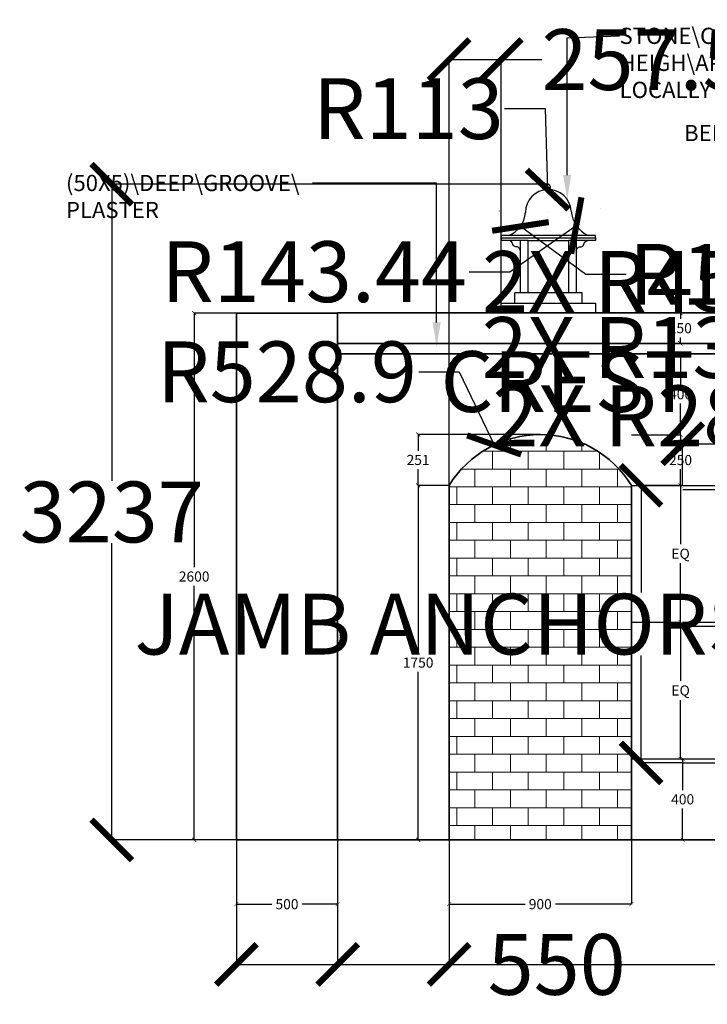
# Model space of a CAD drawing. Units: millimetres. Extents: x 16635 to 28332, y 17519 to 22633.
# Tile 1 of 4: x 16635 to 20029, y 17772 to 22633. Entities that reach past the tile are written whole.
import ezdxf
from ezdxf import colors
from ezdxf.entities.mleader import LeaderData, LeaderLine
from ezdxf.math import Vec2, Vec3

# ---------------------------------------------------------------- set-up
doc = ezdxf.new("R2010")
doc.units = ezdxf.units.MM
doc.header["$MEASUREMENT"] = 0
for name, color, linetype, lineweight in [('A-ANNO-DIMS', 2, 'Continuous', 18), ('A-ANNO-TEXT', 7, 'Continuous', 18), ('A-GATE-HRDW', 3, 'Continuous', 25), ('A-WALL', 7, 'Continuous', 35), ('A-WALL-CHTR', 32, 'Continuous', 25), ('A-WALL-PATT', 8, 'Continuous', 13)]:
    doc.layers.add(name, color=color, linetype=linetype, lineweight=lineweight)
doc.styles.get("Standard").update_dxf_attribs({"font": 'arial.ttf'})
doc.dimstyles.get("Standard").update_dxf_attribs({"dimtxt": 300, "dimasz": 200, "dimexe": 0.18, "dimexo": 0.0625, "dimgap": 0.09, "dimtad": 0, "dimtih": 1, "dimtoh": 1, "dimdec": 0, "dimzin": 0, "dimdsep": 46, "dimtxsty": 'Standard', "dimblk": 'ARCHTICK', "dimcen": 0.09, "dimadec": 0, "dimazin": 0, "dimtfac": 1, "dimtdec": 0, "dimtofl": 0, "dimtmove": 0, "dimatfit": 3, "dimfxl": 1, "dimtolj": 1, "dimtzin": 0, "dimarcsym": 0})

# ---------------------------------------------------------------- blocks, each defined once
blk = doc.blocks.new('_ArchTick')
at = {"color": 0, "linetype": 'ByBlock', "const_width": 0.15}
blk.add_lwpolyline([(-0.5, -0.5), (0.5, 0.5)], dxfattribs=at)
blk = doc.blocks.new('*D9')
at = {"layer": 'A-ANNO-DIMS', "color": 0, "lineweight": -2, "transparency": 16777216}
for p, q in [((18754.7, 20334.3), (18601.7, 20334.3)), ((18601.9, 20334.3), (18601.9, 19504.9)), ((18601.9, 18584.3), (18601.9, 19413.8)), ((18754.7, 18584.3), (18601.7, 18584.3))]:
    blk.add_line(p, q, dxfattribs=at)
at = {"layer": 'Defpoints', "color": 0, "transparency": 16777216}
for p in [(18754.8, 20334.3), (18601.9, 18584.3), (18754.8, 18584.3)]:
    blk.add_point(p, dxfattribs=at)
at = {"layer": 'A-ANNO-DIMS', "color": 0, "lineweight": -2, "transparency": 16777216, "xscale": 20, "yscale": 20, "zscale": 20}
for p, rotation in [((18601.9, 20334.3), 90), ((18601.9, 18584.3), 270)]:
    blk.add_blockref('_ArchTick', p, dxfattribs=dict(at, rotation=rotation))
at = {"layer": 'A-ANNO-DIMS', "color": 0, "transparency": 16777216, "insert": (18601.9, 19459.3), "char_height": 50, "attachment_point": 5}
blk.add_mtext('\\A1;1750', dxfattribs=at)
blk = doc.blocks.new('*D10')
at = {"layer": 'A-ANNO-DIMS', "color": 0, "lineweight": -2, "transparency": 16777216}
for p, q in [((19204.7, 20585.3), (18601.7, 20585.3)), ((18601.9, 20585.3), (18601.9, 20505.4)), ((18601.9, 20334.3), (18601.9, 20414.3)), ((18754.7, 20334.3), (18601.7, 20334.3))]:
    blk.add_line(p, q, dxfattribs=at)
at = {"layer": 'Defpoints', "color": 0, "transparency": 16777216}
for p in [(18601.9, 20585.3), (19204.8, 20585.3), (18754.8, 20334.3)]:
    blk.add_point(p, dxfattribs=at)
at = {"layer": 'A-ANNO-DIMS', "color": 0, "lineweight": -2, "transparency": 16777216, "xscale": 20, "yscale": 20, "zscale": 20}
for p, rotation in [((18601.9, 20585.3), 90), ((18601.9, 20334.3), 270)]:
    blk.add_blockref('_ArchTick', p, dxfattribs=dict(at, rotation=rotation))
at = {"layer": 'A-ANNO-DIMS', "color": 0, "transparency": 16777216, "insert": (18601.9, 20459.8), "char_height": 50, "attachment_point": 5}
blk.add_mtext('\\A1;251', dxfattribs=at)
blk = doc.blocks.new('*D11')
at = {"layer": 'A-ANNO-DIMS', "color": 0, "lineweight": -2, "transparency": 16777216}
for p, q in [((19654.8, 20584.3), (19897.4, 20584.3)), ((19897.2, 20584.3), (19897.2, 20504.9)), ((19897.2, 20334.3), (19897.2, 20413.8)), ((19654.8, 20334.3), (19897.4, 20334.3))]:
    blk.add_line(p, q, dxfattribs=at)
at = {"layer": 'Defpoints', "color": 0, "transparency": 16777216}
for p in [(19654.8, 20584.3), (19897.2, 20584.3), (19654.8, 20334.3)]:
    blk.add_point(p, dxfattribs=at)
at = {"layer": 'A-ANNO-DIMS', "color": 0, "lineweight": -2, "transparency": 16777216, "xscale": 20, "yscale": 20, "zscale": 20}
for p, rotation in [((19897.2, 20584.3), 90), ((19897.2, 20334.3), 270)]:
    blk.add_blockref('_ArchTick', p, dxfattribs=dict(at, rotation=rotation))
at = {"layer": 'A-ANNO-DIMS', "color": 0, "transparency": 16777216, "insert": (19897.2, 20459.3), "char_height": 50, "attachment_point": 5}
blk.add_mtext('\\A1;250', dxfattribs=at)
blk = doc.blocks.new('*D12')
at = {"layer": 'A-ANNO-DIMS', "color": 0, "lineweight": -2, "transparency": 16777216}
for p, q in [((19654.8, 20984.3), (19897.6, 20984.3)), ((19897.4, 20984.3), (19897.4, 20829.9)), ((19897.4, 20584.3), (19897.4, 20738.8)), ((19654.8, 20584.3), (19897.6, 20584.3))]:
    blk.add_line(p, q, dxfattribs=at)
at = {"layer": 'Defpoints', "color": 0, "transparency": 16777216}
for p in [(19654.8, 20984.3), (19897.4, 20984.3), (19654.8, 20584.3)]:
    blk.add_point(p, dxfattribs=at)
at = {"layer": 'A-ANNO-DIMS', "color": 0, "lineweight": -2, "transparency": 16777216, "xscale": 20, "yscale": 20, "zscale": 20}
for p, rotation in [((19897.4, 20984.3), 90), ((19897.4, 20584.3), 270)]:
    blk.add_blockref('_ArchTick', p, dxfattribs=dict(at, rotation=rotation))
at = {"layer": 'A-ANNO-DIMS', "color": 0, "transparency": 16777216, "insert": (19897.4, 20784.3), "char_height": 50, "attachment_point": 5}
blk.add_mtext('\\A1;400', dxfattribs=at)
blk = doc.blocks.new('*D18')
at = {"layer": 'A-ANNO-DIMS', "color": 0, "lineweight": -2, "transparency": 16777216}
for p, q in [((17704.7, 21184.3), (17496.3, 21184.3)), ((17496.5, 21184.3), (17496.5, 19929.9)), ((17496.5, 18584.3), (17496.5, 19838.8)), ((17704.7, 18584.3), (17496.3, 18584.3))]:
    blk.add_line(p, q, dxfattribs=at)
at = {"layer": 'Defpoints', "color": 0, "transparency": 16777216}
for p in [(17704.8, 21184.3), (17496.5, 18584.3), (17704.8, 18584.3)]:
    blk.add_point(p, dxfattribs=at)
at = {"layer": 'A-ANNO-DIMS', "color": 0, "lineweight": -2, "transparency": 16777216, "xscale": 20, "yscale": 20, "zscale": 20}
for p, rotation in [((17496.5, 21184.3), 90), ((17496.5, 18584.3), 270)]:
    blk.add_blockref('_ArchTick', p, dxfattribs=dict(at, rotation=rotation))
at = {"layer": 'A-ANNO-DIMS', "color": 0, "transparency": 16777216, "insert": (17496.5, 19884.3), "char_height": 50, "attachment_point": 5}
blk.add_mtext('\\A1;2600', dxfattribs=at)
blk = doc.blocks.new('*D23')
at = {"layer": 'A-ANNO-DIMS', "color": 0, "lineweight": -2, "transparency": 16777216}
for p, q in [((18754.8, 18584.3), (18754.8, 18266.8)), ((19654.8, 18584.3), (19654.8, 18266.8)), ((18754.8, 18267), (19129.6, 18267)), ((19654.8, 18267), (19279.9, 18267))]:
    blk.add_line(p, q, dxfattribs=at)
at = {"layer": 'Defpoints', "color": 0, "transparency": 16777216}
for p in [(18754.8, 18584.3), (19654.8, 18584.3), (19654.8, 18267)]:
    blk.add_point(p, dxfattribs=at)
at = {"layer": 'A-ANNO-DIMS', "color": 0, "lineweight": -2, "transparency": 16777216, "xscale": 20, "yscale": 20, "zscale": 20, "rotation": 180}
blk.add_blockref('_ArchTick', (18754.8, 18267), dxfattribs=at)
at = {"layer": 'A-ANNO-DIMS', "color": 0, "lineweight": -2, "transparency": 16777216, "xscale": 20, "yscale": 20, "zscale": 20}
blk.add_blockref('_ArchTick', (19654.8, 18267), dxfattribs=at)
at = {"layer": 'A-ANNO-DIMS', "color": 0, "transparency": 16777216, "insert": (19204.8, 18267), "char_height": 50, "attachment_point": 5}
blk.add_mtext('\\A1;900', dxfattribs=at)
blk = doc.blocks.new('*D24')
at = {"layer": 'A-ANNO-DIMS', "color": 0, "lineweight": -2, "transparency": 16777216}
for p, q in [((17704.8, 18584.3), (17704.8, 18266.6)), ((18204.8, 18584.3), (18204.8, 18266.6)), ((17704.8, 18266.8), (17879.6, 18266.8)), ((18204.8, 18266.8), (18029.9, 18266.8))]:
    blk.add_line(p, q, dxfattribs=at)
at = {"layer": 'Defpoints', "color": 0, "transparency": 16777216}
for p in [(17704.8, 18584.3), (18204.8, 18584.3), (18204.8, 18266.8)]:
    blk.add_point(p, dxfattribs=at)
at = {"layer": 'A-ANNO-DIMS', "color": 0, "lineweight": -2, "transparency": 16777216, "xscale": 20, "yscale": 20, "zscale": 20, "rotation": 180}
blk.add_blockref('_ArchTick', (17704.8, 18266.8), dxfattribs=at)
at = {"layer": 'A-ANNO-DIMS', "color": 0, "lineweight": -2, "transparency": 16777216, "xscale": 20, "yscale": 20, "zscale": 20}
blk.add_blockref('_ArchTick', (18204.8, 18266.8), dxfattribs=at)
at = {"layer": 'A-ANNO-DIMS', "color": 0, "transparency": 16777216, "insert": (17954.8, 18266.8), "char_height": 50, "attachment_point": 5}
blk.add_mtext('\\A1;500', dxfattribs=at)
blk = doc.blocks.new('*D31')
at = {"layer": 'A-ANNO-DIMS', "color": 0, "lineweight": -2, "transparency": 16777216}
for p, q in [((19654.8, 18984.3), (19907.7, 18984.3)), ((19907.6, 18984.3), (19907.6, 18829.9)), ((19907.6, 18584.3), (19907.6, 18738.8)), ((19654.8, 18584.3), (19907.7, 18584.3))]:
    blk.add_line(p, q, dxfattribs=at)
at = {"layer": 'Defpoints', "color": 0, "transparency": 16777216}
for p in [(19654.8, 18984.3), (19907.6, 18984.3), (19654.8, 18584.3)]:
    blk.add_point(p, dxfattribs=at)
at = {"layer": 'A-ANNO-DIMS', "color": 0, "lineweight": -2, "transparency": 16777216, "xscale": 20, "yscale": 20, "zscale": 20}
for p, rotation in [((19907.6, 18984.3), 90), ((19907.6, 18584.3), 270)]:
    blk.add_blockref('_ArchTick', p, dxfattribs=dict(at, rotation=rotation))
at = {"layer": 'A-ANNO-DIMS', "color": 0, "transparency": 16777216, "insert": (19907.6, 18784.3), "char_height": 50, "attachment_point": 5}
blk.add_mtext('\\A1;400', dxfattribs=at)
blk = doc.blocks.new('*D35')
at = {"layer": 'A-ANNO-DIMS', "color": 0, "lineweight": -2, "transparency": 16777216}
for p, q in [((19654.8, 20334.3), (19897.6, 20334.3)), ((19897.4, 20334.3), (19897.4, 20044.2)), ((19897.4, 19659.3), (19897.4, 19949.5)), ((19654.8, 19659.3), (19897.6, 19659.3))]:
    blk.add_line(p, q, dxfattribs=at)
at = {"layer": 'Defpoints', "color": 0, "transparency": 16777216}
for p in [(19654.8, 20334.3), (19654.8, 19659.3), (19897.4, 19659.3)]:
    blk.add_point(p, dxfattribs=at)
at = {"layer": 'A-ANNO-DIMS', "color": 0, "lineweight": -2, "transparency": 16777216, "xscale": 20, "yscale": 20, "zscale": 20}
for p, rotation in [((19897.4, 20334.3), 90), ((19897.4, 19659.3), 270)]:
    blk.add_blockref('_ArchTick', p, dxfattribs=dict(at, rotation=rotation))
at = {"layer": 'A-ANNO-DIMS', "color": 0, "transparency": 16777216, "insert": (19897.4, 19996.8), "char_height": 50, "attachment_point": 5}
blk.add_mtext('\\A1;EQ', dxfattribs=at)
blk = doc.blocks.new('*D36')
at = {"layer": 'A-ANNO-DIMS', "color": 0, "lineweight": -2, "transparency": 16777216}
for p, q in [((19654.8, 19659.3), (19897.7, 19659.3)), ((19897.6, 19659.3), (19897.6, 19369.2)), ((19897.6, 18984.3), (19897.6, 19274.5)), ((19654.8, 18984.3), (19897.7, 18984.3))]:
    blk.add_line(p, q, dxfattribs=at)
at = {"layer": 'Defpoints', "color": 0, "transparency": 16777216}
for p in [(19654.8, 19659.3), (19654.8, 18984.3), (19897.6, 18984.3)]:
    blk.add_point(p, dxfattribs=at)
at = {"layer": 'A-ANNO-DIMS', "color": 0, "lineweight": -2, "transparency": 16777216, "xscale": 20, "yscale": 20, "zscale": 20}
for p, rotation in [((19897.6, 19659.3), 90), ((19897.6, 18984.3), 270)]:
    blk.add_blockref('_ArchTick', p, dxfattribs=dict(at, rotation=rotation))
at = {"layer": 'A-ANNO-DIMS', "color": 0, "transparency": 16777216, "insert": (19897.6, 19321.8), "char_height": 50, "attachment_point": 5}
blk.add_mtext('\\A1;EQ', dxfattribs=at)
blk = doc.blocks.new('*D37')
at = {"layer": 'A-ANNO-DIMS', "color": 0, "lineweight": -2, "transparency": 16777216}
for p, q in [((19896.2, 21185.3), (19896.2, 21155.9)), ((19896.3, 21185.3), (19896.4, 21185.3)), ((19896.2, 21035.3), (19896.2, 21064.8)), ((19896.3, 21035.3), (19896.4, 21035.3))]:
    blk.add_line(p, q, dxfattribs=at)
at = {"layer": 'Defpoints', "color": 0, "transparency": 16777216}
for p in [(19896.2, 21185.3), (19896.2, 21185.3), (19896.2, 21035.3)]:
    blk.add_point(p, dxfattribs=at)
at = {"layer": 'A-ANNO-DIMS', "color": 0, "lineweight": -2, "transparency": 16777216, "xscale": 20, "yscale": 20, "zscale": 20}
for p, rotation in [((19896.2, 21185.3), 90), ((19896.2, 21035.3), 270)]:
    blk.add_blockref('_ArchTick', p, dxfattribs=dict(at, rotation=rotation))
at = {"layer": 'A-ANNO-DIMS', "color": 0, "transparency": 16777216, "insert": (19896.2, 21110.3), "char_height": 50, "attachment_point": 5}
blk.add_mtext('\\A1;150', dxfattribs=at)
blk = doc.blocks.new('STONE-CHHATRI-ELEV')
for p, q in [((465, 384), (0, 384)), ((0, 384), (0, 359)), ((0, 371.5), (465, 371.5)), ((132.5, 359), (0, 359)), ((94.5, 100), (94.5, 359)), ((132.5, 100), (132.5, 359)), ((132.5, 359), (332.5, 359)), ((332.5, 359), (332.5, 100)), ((465, 359), (332.5, 359)), ((370.5, 359), (370.5, 100)), ((465, 371.5), (465, 384)), ((465, 371.5), (465, 359)), ((398.8, 100), (66.3, 100)), ((66.3, 50), (66.3, 100)), ((398.8, 50), (398.8, 100)), ((0, 0), (0, 50)), ((0, 50), (465, 50)), ((465, 50), (465, 0))]:
    blk.add_line(p, q)
for points in [[(223.5, 618.7, -0.258687), (233, 636.9, -0.244698), (241.5, 619.3, -0.244698)], [(94.5, 307.9, 0.449164), (70.8, 327.5, -0.238561), (57.7, 338.5, 0.309009), (37.1, 359, -1.219644)], [(370.5, 307.9, -0.449164), (394.2, 327.5, 0.238561), (407.3, 338.5, -0.309009), (427.9, 359, 1.219644)]]:
    blk.add_lwpolyline(points, format="xyb")
for centre, radius, start, end in [((232.5, 497), 113, 3.6245, 179.9064), ((232.5, 619), 9.02, 180.1799, 1.9928), ((-8.8, 504.3), 128.5, 290.6287, 356.8247), ((488.3, 514.4), 143.4, 184.0947, 245.367)]:
    blk.add_arc(centre, radius, start, end)
blk = doc.blocks.new('GATE-JAMB-ANCHOR-SET')
for p, q in [((0.2, 1370), (297.2, 1370)), ((317.2, 1350), (317.2, 1370)), ((317.2, 1370), (351.9, 1370)), ((0.2, 1350), (297.2, 1350)), ((297.2, 1350), (317.2, 1350)), ((0, 694.8), (297, 694.8)), ((317, 674.8), (317, 694.8)), ((317, 694.8), (365.3, 694.8)), ((0, 674.8), (297, 674.8)), ((297, 674.8), (317, 674.8)), ((0.2, 20), (297.2, 20)), ((317.2, 0), (317.2, 20)), ((317.2, 20), (360.9, 20)), ((0.2, 0), (297.2, 0)), ((297.2, 0), (317.2, 0))]:
    blk.add_line(p, q)
blk = doc.blocks.new('*D47')
at = {"layer": 'A-ANNO-DIMS', "color": 0, "lineweight": -2, "transparency": 16777216}
for p, q in [((21092.8, 21187.8), (20990.3, 21187.8)), ((20990.5, 21187.8), (20990.5, 21001.9)), ((20990.5, 20505.3), (20990.5, 20691.3)), ((21092.8, 20505.3), (20990.3, 20505.3))]:
    blk.add_line(p, q, dxfattribs=at)
at = {"layer": 'Defpoints', "color": 0, "transparency": 16777216}
for p in [(20990.5, 21187.8), (21092.8, 21187.8), (21092.8, 20505.3)]:
    blk.add_point(p, dxfattribs=at)
at = {"layer": 'A-ANNO-DIMS', "color": 0, "lineweight": -2, "transparency": 16777216, "xscale": 200, "yscale": 200, "zscale": 200}
for p, rotation in [((20990.5, 21187.8), 90), ((20990.5, 20505.3), 270)]:
    blk.add_blockref('_ArchTick', p, dxfattribs=dict(at, rotation=rotation))
at = {"layer": 'A-ANNO-DIMS', "color": 0, "transparency": 16777216, "insert": (20990.5, 20846.6), "char_height": 300, "attachment_point": 5}
blk.add_mtext('\\A1;CREST SCROLL 682 TYP.', dxfattribs=at)
blk = doc.blocks.new('*D49')
at = {"layer": 'A-ANNO-DIMS', "color": 0, "lineweight": -2, "transparency": 16777216}
for p, q in [((19907.5, 20334.3), (19701.9, 20334.3)), ((19702.1, 20334.3), (19702.1, 19804.8)), ((19702.1, 18964.3), (19702.1, 19493.9)), ((19907.5, 18964.3), (19701.9, 18964.3))]:
    blk.add_line(p, q, dxfattribs=at)
at = {"layer": 'Defpoints', "color": 0, "transparency": 16777216}
for p in [(19702.1, 20334.3), (19907.6, 20334.3), (19907.6, 18964.3)]:
    blk.add_point(p, dxfattribs=at)
at = {"layer": 'A-ANNO-DIMS', "color": 0, "lineweight": -2, "transparency": 16777216, "xscale": 200, "yscale": 200, "zscale": 200}
for p, rotation in [((19702.1, 20334.3), 90), ((19702.1, 18964.3), 270)]:
    blk.add_blockref('_ArchTick', p, dxfattribs=dict(at, rotation=rotation))
at = {"layer": 'A-ANNO-DIMS', "color": 0, "transparency": 16777216, "insert": (19702.1, 19649.3), "char_height": 300, "attachment_point": 5}
blk.add_mtext('\\A1;JAMB ANCHORS 1370 TYP.', dxfattribs=at)
blk = doc.blocks.new('*D50')
at = {"layer": 'A-ANNO-DIMS', "color": 0, "lineweight": -2, "transparency": 16777216}
for p, q in [((19907.6, 20334.4), (19907.6, 20540)), ((19907.6, 20539.8), (20272.8, 20539.8)), ((20272.8, 20334.4), (20272.8, 20540)), ((20272.8, 20539.8), (20472.8, 20539.8))]:
    blk.add_line(p, q, dxfattribs=at)
at = {"layer": 'Defpoints', "color": 0, "transparency": 16777216}
for p in [(20272.8, 20539.8), (19907.6, 20334.3), (20272.8, 20334.3)]:
    blk.add_point(p, dxfattribs=at)
at = {"layer": 'A-ANNO-DIMS', "color": 0, "lineweight": -2, "transparency": 16777216, "xscale": 200, "yscale": 200, "zscale": 200, "rotation": 180}
blk.add_blockref('_ArchTick', (19907.6, 20539.8), dxfattribs=at)
at = {"layer": 'A-ANNO-DIMS', "color": 0, "lineweight": -2, "transparency": 16777216, "xscale": 200, "yscale": 200, "zscale": 200}
blk.add_blockref('_ArchTick', (20272.8, 20539.8), dxfattribs=at)
at = {"layer": 'A-ANNO-DIMS', "color": 0, "transparency": 16777216, "insert": (21319.5, 20539.8), "char_height": 300, "attachment_point": 5}
blk.add_mtext('\\A1;365 TYP.', dxfattribs=at)
blk = doc.blocks.new('*D51')
at = {"layer": 'A-ANNO-DIMS', "color": 0, "lineweight": -2, "transparency": 16777216}
for p, q in [((17704.8, 18584.3), (17704.8, 17969.2)), ((26604.8, 18584.3), (26604.8, 17969.2)), ((17704.8, 17969.3), (21707, 17969.3)), ((26604.8, 17969.3), (22602.5, 17969.3))]:
    blk.add_line(p, q, dxfattribs=at)
at = {"layer": 'Defpoints', "color": 0, "transparency": 16777216}
for p in [(17704.8, 18584.3), (26604.8, 18584.3), (26604.8, 17969.3)]:
    blk.add_point(p, dxfattribs=at)
at = {"layer": 'A-ANNO-DIMS', "color": 0, "lineweight": -2, "transparency": 16777216, "xscale": 200, "yscale": 200, "zscale": 200, "rotation": 180}
blk.add_blockref('_ArchTick', (17704.8, 17969.3), dxfattribs=at)
at = {"layer": 'A-ANNO-DIMS', "color": 0, "lineweight": -2, "transparency": 16777216, "xscale": 200, "yscale": 200, "zscale": 200}
blk.add_blockref('_ArchTick', (26604.8, 17969.3), dxfattribs=at)
at = {"layer": 'A-ANNO-DIMS', "color": 0, "transparency": 16777216, "insert": (22154.8, 17969.3), "char_height": 300, "attachment_point": 5}
blk.add_mtext('\\A1;8900', dxfattribs=at)
blk = doc.blocks.new('*D52')
at = {"layer": 'A-ANNO-DIMS', "color": 0, "lineweight": -2, "transparency": 16777216}
for p, q in [((19245.2, 21821.2), (17089.6, 21821.2)), ((17089.8, 21821.2), (17089.8, 20356.2)), ((17089.8, 18584.3), (17089.8, 20049.4)), ((18754.7, 18584.3), (17089.6, 18584.3))]:
    blk.add_line(p, q, dxfattribs=at)
at = {"layer": 'Defpoints', "color": 0, "transparency": 16777216}
for p in [(17089.8, 21821.2), (19245.2, 21821.2), (18754.8, 18584.3)]:
    blk.add_point(p, dxfattribs=at)
at = {"layer": 'A-ANNO-DIMS', "color": 0, "lineweight": -2, "transparency": 16777216, "xscale": 200, "yscale": 200, "zscale": 200}
for p, rotation in [((17089.8, 21821.2), 90), ((17089.8, 18584.3), 270)]:
    blk.add_blockref('_ArchTick', p, dxfattribs=dict(at, rotation=rotation))
at = {"layer": 'A-ANNO-DIMS', "color": 0, "transparency": 16777216, "insert": (17089.8, 20202.8), "char_height": 300, "attachment_point": 5}
blk.add_mtext('\\A1;3237', dxfattribs=at)
blk = doc.blocks.new('*D53')
at = {"layer": 'A-ANNO-DIMS', "color": 0, "lineweight": -2, "transparency": 16777216}
for p, q in [((18204.8, 18584.3), (18204.8, 17969.2)), ((18754.8, 18584.3), (18754.8, 17969.2)), ((18204.8, 17969.3), (18754.8, 17969.3)), ((18754.8, 17969.3), (18954.8, 17969.3))]:
    blk.add_line(p, q, dxfattribs=at)
at = {"layer": 'Defpoints', "color": 0, "transparency": 16777216}
for p in [(18204.8, 18584.3), (18754.8, 18584.3), (18754.8, 17969.3)]:
    blk.add_point(p, dxfattribs=at)
at = {"layer": 'A-ANNO-DIMS', "color": 0, "lineweight": -2, "transparency": 16777216, "xscale": 200, "yscale": 200, "zscale": 200, "rotation": 180}
blk.add_blockref('_ArchTick', (18204.8, 17969.3), dxfattribs=at)
at = {"layer": 'A-ANNO-DIMS', "color": 0, "lineweight": -2, "transparency": 16777216, "xscale": 200, "yscale": 200, "zscale": 200}
blk.add_blockref('_ArchTick', (18754.8, 17969.3), dxfattribs=at)
at = {"layer": 'A-ANNO-DIMS', "color": 0, "transparency": 16777216, "insert": (19285.8, 17969.3), "char_height": 300, "attachment_point": 5}
blk.add_mtext('\\A1;550', dxfattribs=at)
blk = doc.blocks.new('*D59')
at = {"layer": 'A-ANNO-DIMS', "color": 0, "lineweight": -2, "transparency": 16777216}
for p, q in [((18754.8, 20334.4), (18754.8, 22436.4)), ((18754.8, 22436.2), (19012.3, 22436.2)), ((19012.3, 21184.4), (19012.3, 22436.4)), ((19012.3, 22436.2), (19212.3, 22436.2))]:
    blk.add_line(p, q, dxfattribs=at)
at = {"layer": 'Defpoints', "color": 0, "transparency": 16777216}
for p in [(19012.3, 22436.2), (19012.3, 21184.3), (18754.8, 20334.3)]:
    blk.add_point(p, dxfattribs=at)
at = {"layer": 'A-ANNO-DIMS', "color": 0, "lineweight": -2, "transparency": 16777216, "xscale": 200, "yscale": 200, "zscale": 200, "rotation": 180}
blk.add_blockref('_ArchTick', (18754.8, 22436.2), dxfattribs=at)
at = {"layer": 'A-ANNO-DIMS', "color": 0, "lineweight": -2, "transparency": 16777216, "xscale": 200, "yscale": 200, "zscale": 200}
blk.add_blockref('_ArchTick', (19012.3, 22436.2), dxfattribs=at)
at = {"layer": 'A-ANNO-DIMS', "color": 0, "transparency": 16777216, "insert": (19722.2, 22436.2), "char_height": 300, "attachment_point": 5}
blk.add_mtext('\\A1;257.5', dxfattribs=at)
blk = doc.blocks.new('*D62')
at = {"layer": 'A-ANNO-DIMS', "color": 0, "lineweight": -2, "transparency": 16777216}
for p, q in [((18604.9, 20894.9), (18804.9, 20894.9)), ((18804.9, 20894.9), (18977.1, 20533.8)), ((19204.7, 20056.5), (19204.9, 20056.5)), ((19204.8, 20056.4), (19204.8, 20056.6))]:
    blk.add_line(p, q, dxfattribs=at)
at = {"layer": 'Defpoints', "color": 0, "transparency": 16777216}
for p in [(18977.1, 20533.8), (19204.8, 20056.5)]:
    blk.add_point(p, dxfattribs=at)
at = {"layer": 'A-ANNO-DIMS', "color": 0, "lineweight": -2, "transparency": 16777216, "xscale": 200, "yscale": 200, "zscale": 200, "rotation": 295.4996484836518}
blk.add_blockref('_ArchTick', (18977.1, 20533.8), dxfattribs=at)
at = {"layer": 'A-ANNO-DIMS', "color": 0, "transparency": 16777216, "insert": (17954.8, 20894.9), "char_height": 300, "attachment_point": 5}
blk.add_mtext('\\A1;R528.9', dxfattribs=at)
blk = doc.blocks.new('*D64')
at = {"layer": 'A-ANNO-DIMS', "color": 0, "lineweight": -2, "transparency": 16777216}
for p, q in [((19029, 22194.1), (19229, 22194.1)), ((19229, 22194.1), (19241.3, 21794.3)), ((19244.7, 21681.3), (19244.9, 21681.3)), ((19244.8, 21681.3), (19244.8, 21681.4))]:
    blk.add_line(p, q, dxfattribs=at)
at = {"layer": 'Defpoints', "color": 0, "transparency": 16777216}
for p in [(19241.3, 21794.3), (19244.8, 21681.3)]:
    blk.add_point(p, dxfattribs=at)
at = {"layer": 'A-ANNO-DIMS', "color": 0, "lineweight": -2, "transparency": 16777216, "xscale": 200, "yscale": 200, "zscale": 200, "rotation": 271.765444165323}
blk.add_blockref('_ArchTick', (19241.3, 21794.3), dxfattribs=at)
at = {"layer": 'A-ANNO-DIMS', "color": 0, "transparency": 16777216, "insert": (18553.9, 22194.1), "char_height": 300, "attachment_point": 5}
blk.add_mtext('\\A1;R113', dxfattribs=at)
blk = doc.blocks.new('*D65')
at = {"layer": 'A-ANNO-DIMS', "color": 0, "lineweight": -2, "transparency": 16777216}
for p, q in [((19500.5, 21698.7), (19500.7, 21698.7)), ((19500.6, 21698.6), (19500.6, 21698.8)), ((19054, 21389.1), (19382.7, 21617)), ((18854, 21389.1), (19054, 21389.1))]:
    blk.add_line(p, q, dxfattribs=at)
at = {"layer": 'Defpoints', "color": 0, "transparency": 16777216}
for p in [(19500.6, 21698.7), (19382.7, 21617)]:
    blk.add_point(p, dxfattribs=at)
at = {"layer": 'A-ANNO-DIMS', "color": 0, "lineweight": -2, "transparency": 16777216, "xscale": 200, "yscale": 200, "zscale": 200, "rotation": 34.73087780623892}
blk.add_blockref('_ArchTick', (19382.7, 21617), dxfattribs=at)
at = {"layer": 'A-ANNO-DIMS', "color": 0, "transparency": 16777216, "insert": (18088.3, 21389.1), "char_height": 300, "attachment_point": 5}
blk.add_mtext('\\A1;R143.44', dxfattribs=at)
blk = doc.blocks.new('*D66')
at = {"layer": 'A-ANNO-DIMS', "color": 0, "lineweight": -2, "transparency": 16777216}
for p, q in [((19003.3, 21688.7), (19003.5, 21688.7)), ((19003.4, 21688.6), (19003.4, 21688.7)), ((19429.5, 21375.9), (19107.1, 21612.6)), ((19629.5, 21375.9), (19429.5, 21375.9))]:
    blk.add_line(p, q, dxfattribs=at)
at = {"layer": 'Defpoints', "color": 0, "transparency": 16777216}
for p in [(19003.4, 21688.7), (19107.1, 21612.6)]:
    blk.add_point(p, dxfattribs=at)
at = {"layer": 'A-ANNO-DIMS', "color": 0, "lineweight": -2, "transparency": 16777216, "xscale": 200, "yscale": 200, "zscale": 200, "rotation": 143.726603085954}
blk.add_blockref('_ArchTick', (19107.1, 21612.6), dxfattribs=at)
at = {"layer": 'A-ANNO-DIMS', "color": 0, "transparency": 16777216, "insert": (20397, 21375.9), "char_height": 300, "attachment_point": 5}
blk.add_mtext('\\A1;R128.55', dxfattribs=at)
blk = doc.blocks.new('*D69')
at = {"layer": 'A-ANNO-DIMS', "color": 0, "lineweight": -2, "transparency": 16777216}
for p, q in [((20810.7, 21340.9), (21010.7, 21340.9)), ((21010.7, 21340.9), (21090, 20948.9)), ((21179.7, 20505.3), (21179.9, 20505.3)), ((21179.8, 20505.3), (21179.8, 20505.4))]:
    blk.add_line(p, q, dxfattribs=at)
at = {"layer": 'Defpoints', "color": 0, "transparency": 16777216}
for p in [(21090, 20948.9), (21179.8, 20505.3)]:
    blk.add_point(p, dxfattribs=at)
at = {"layer": 'A-ANNO-DIMS', "color": 0, "lineweight": -2, "transparency": 16777216, "xscale": 200, "yscale": 200, "zscale": 200, "rotation": 281.4390211623567}
blk.add_blockref('_ArchTick', (21090, 20948.9), dxfattribs=at)
at = {"layer": 'A-ANNO-DIMS', "color": 0, "transparency": 16777216, "insert": (19834.9, 21340.9), "char_height": 300, "attachment_point": 5}
blk.add_mtext('\\A1;2X R452.5', dxfattribs=at)
blk = doc.blocks.new('*D72')
at = {"layer": 'A-ANNO-DIMS', "color": 0, "lineweight": -2, "transparency": 16777216}
for p, q in [((20516.7, 20677.3), (20903.9, 20576.9)), ((21179.7, 20505.3), (21179.9, 20505.3)), ((21179.8, 20505.3), (21179.8, 20505.4))]:
    blk.add_line(p, q, dxfattribs=at)
at = {"layer": 'Defpoints', "color": 0, "transparency": 16777216}
for p in [(20903.9, 20576.9), (21179.8, 20505.3)]:
    blk.add_point(p, dxfattribs=at)
at = {"layer": 'A-ANNO-DIMS', "color": 0, "lineweight": -2, "transparency": 16777216, "xscale": 200, "yscale": 200, "zscale": 200, "rotation": 345.4648454983082}
blk.add_blockref('_ArchTick', (20903.9, 20576.9), dxfattribs=at)
at = {"layer": 'A-ANNO-DIMS', "color": 0, "transparency": 16777216, "insert": (19715.6, 20677.3), "char_height": 300, "attachment_point": 5}
blk.add_mtext('\\A1;2X R285', dxfattribs=at)
blk = doc.blocks.new('*D74')
at = {"layer": 'A-ANNO-DIMS', "color": 0, "lineweight": -2, "transparency": 16777216}
for p, q in [((20809, 21015), (21009, 21015)), ((21009, 21015), (21136.1, 20635.7)), ((21179.7, 20505.3), (21179.9, 20505.3)), ((21179.8, 20505.3), (21179.8, 20505.4))]:
    blk.add_line(p, q, dxfattribs=at)
at = {"layer": 'Defpoints', "color": 0, "transparency": 16777216}
for p in [(21136.1, 20635.7), (21179.8, 20505.3)]:
    blk.add_point(p, dxfattribs=at)
at = {"layer": 'A-ANNO-DIMS', "color": 0, "lineweight": -2, "transparency": 16777216, "xscale": 200, "yscale": 200, "zscale": 200, "rotation": 288.5216632841473}
blk.add_blockref('_ArchTick', (21136.1, 20635.7), dxfattribs=at)
at = {"layer": 'A-ANNO-DIMS', "color": 0, "transparency": 16777216, "insert": (19833.2, 21015), "char_height": 300, "attachment_point": 5}
blk.add_mtext('\\A1;2X R137.5', dxfattribs=at)

msp = doc.modelspace()

# ---------------------------------------------------------------- hatches: boundary and pattern name
at = {"layer": 'A-WALL-PATT'}
h = msp.add_hatch(dxfattribs=at)
h.set_pattern_fill('AR-B816', color=256, scale=11)
h.set_pattern_definition([(0, (15185.615, 17862.945), (0, 88), []), (90, (15185.615, 17862.945), (-88, 88), [88, -88])])
h.paths.add_polyline_path([(19654.77, 20334.349, 0.55777778), (18754.77, 20334.349), (18754.77, 18584.349), (19654.77, 18584.349)])

# ---------------------------------------------------------------- linework, layer by layer
at = {"layer": 'A-WALL'}
for p, q in [((20204.77, 21185.349), (18204.77, 21185.349)), ((20204.77, 21035.349), (18204.77, 21035.349)), ((20204.77, 20984.349), (18204.77, 20984.349)), ((18754.77, 18584.349), (18754.77, 20334.349)), ((19654.77, 18584.349), (19654.77, 20334.349)), ((19654.77, 20334.349), (19654.77, 18984.349)), ((18204.77, 18584.349), (20204.77, 18584.349))]:
    msp.add_line(p, q, dxfattribs=at)
msp.add_lwpolyline([(18204.77, 21184.349), (18204.77, 18584.349), (17704.77, 18584.349), (17704.77, 21184.349)], close=True, dxfattribs=at)
msp.add_arc((19204.77, 20056.462), 528.886, 31.696386, 148.303614, dxfattribs=at)

# ---------------------------------------------------------------- block references
at = {"layer": 'A-GATE-HRDW'}
msp.add_blockref('GATE-JAMB-ANCHOR-SET', (19907.57, 18964.349), dxfattribs=at)
at = {"layer": 'A-WALL-CHTR'}
msp.add_blockref('STONE-CHHATRI-ELEV', (19012.27, 21184.349), dxfattribs=at)

# ---------------------------------------------------------------- dimensions: what is measured, and where the dimension line sits
at = {"layer": 'A-ANNO-DIMS'}
for base, p1, p2, override, picture, middle in [((19012.27, 22436.24), (18754.77, 20334.349), (19012.27, 21184.349), {"dimdec": 1, "dimlfac": 1, "dimrnd": 0, "dimzin": 0, "dimdsep": 46, "dimlunit": 2}, '*D59', (19722.217, 22436.24)), ((26604.77, 17969.349), (17704.77, 18584.349), (26604.77, 18584.349), {"dimdec": 0, "dimlfac": 1, "dimrnd": 0, "dimzin": 0, "dimdsep": 46, "dimlunit": 2}, '*D51', (22154.77, 17969.349)), ((18204.77, 18266.798), (17704.77, 18584.349), (18204.77, 18584.349), {"dimtxt": 50, "dimasz": 20, "dimgap": 20, "dimclrd": 0, "dimclre": 0, "dimclrt": 0}, '*D24', (17954.77, 18266.798)), ((18754.77, 17969.349), (18204.77, 18584.349), (18754.77, 18584.349), {"dimdec": 0, "dimlfac": 1, "dimrnd": 0, "dimzin": 0, "dimdsep": 46, "dimlunit": 2}, '*D53', (19285.761, 17969.349)), ((19654.77, 18266.978), (18754.77, 18584.349), (19654.77, 18584.349), {"dimtxt": 50, "dimasz": 20, "dimgap": 20, "dimclrd": 0, "dimclre": 0, "dimclrt": 0}, '*D23', (19204.77, 18266.978))]:
    dim = msp.add_linear_dim(base=base, p1=p1, p2=p2, dimstyle='Standard', override=override, dxfattribs=at)
    dim.commit()
    dim.dimension.update_dxf_attribs({"geometry": picture, "text_midpoint": middle})
for center, mpoint, override, picture, middle in [((19244.77, 21681.349), (19241.289, 21794.295), {"dimdec": 0, "dimlfac": 1, "dimrnd": 0, "dimzin": 0, "dimdsep": 46, "dimlunit": 2}, '*D64', (18553.91, 22194.105)), ((19500.618, 21698.734), (19382.734, 21617.014), {"dimdec": 2, "dimlfac": 1, "dimrnd": 0, "dimzin": 0, "dimdsep": 46, "dimlunit": 2}, '*D65', (18088.254, 21389.125)), ((19003.421, 21688.654), (19107.056, 21612.6), {"dimdec": 2, "dimlfac": 1, "dimrnd": 0, "dimzin": 0, "dimdsep": 46, "dimlunit": 2}, '*D66', (20397.021, 21375.945)), ((19204.77, 20056.462), (18977.082, 20533.829), {"dimdec": 1, "dimlfac": 1, "dimrnd": 0, "dimzin": 0, "dimdsep": 46, "dimlunit": 2}, '*D62', (17954.755, 20894.864))]:
    dim = msp.add_radius_dim(center=center, mpoint=mpoint, dimstyle='Standard', override=override, dxfattribs=at)
    dim.commit()
    dim.dimension.update_dxf_attribs({"geometry": picture, "text_midpoint": middle})
for base, p1, p2, override, picture, middle in [((17089.77, 21821.24), (18754.77, 18584.349), (19245.237, 21821.24), {"dimdec": 0, "dimlfac": 1, "dimrnd": 0, "dimzin": 0, "dimdsep": 46, "dimlunit": 2}, '*D52', (17089.77, 20202.794)), ((19896.209, 21185.349), (19896.209, 21035.349), (19896.209, 21185.349), {"dimtxt": 50, "dimasz": 20, "dimgap": 20, "dimclrd": 0, "dimclre": 0, "dimclrt": 0}, '*D37', (19896.209, 21110.349)), ((19897.39, 20984.349), (19654.77, 20584.349), (19654.77, 20984.349), {"dimtxt": 50, "dimasz": 20, "dimgap": 20, "dimclrd": 0, "dimclre": 0, "dimclrt": 0}, '*D12', (19897.39, 20784.349)), ((18601.918, 20585.349), (18754.77, 20334.349), (19204.77, 20585.349), {"dimtxt": 50, "dimasz": 20, "dimgap": 20, "dimclrd": 0, "dimclre": 0, "dimclrt": 0}, '*D10', (18601.918, 20459.849)), ((19897.21, 20584.349), (19654.77, 20334.349), (19654.77, 20584.349), {"dimtxt": 50, "dimasz": 20, "dimgap": 20, "dimclrd": 0, "dimclre": 0, "dimclrt": 0}, '*D11', (19897.21, 20459.349)), ((18601.918, 18584.349), (18754.77, 20334.349), (18754.77, 18584.349), {"dimtxt": 50, "dimasz": 20, "dimgap": 20, "dimclrd": 0, "dimclre": 0, "dimclrt": 0}, '*D9', (18601.918, 19459.349)), ((19907.57, 18984.349), (19654.77, 18584.349), (19654.77, 18984.349), {"dimtxt": 50, "dimasz": 20, "dimgap": 20, "dimclrd": 0, "dimclre": 0, "dimclrt": 0}, '*D31', (19907.57, 18784.349))]:
    dim = msp.add_linear_dim(base=base, p1=p1, p2=p2, angle=90, dimstyle='Standard', override=override, dxfattribs=at)
    dim.commit()
    dim.dimension.update_dxf_attribs({"geometry": picture, "text_midpoint": middle})
for base, p1, p2, text, override, picture, middle in [((20990.466, 21187.833), (21092.839, 20505.349), (21092.839, 21187.833), 'CREST SCROLL <> TYP.', {"dimdec": 0, "dimlfac": 1, "dimrnd": 0, "dimzin": 0, "dimdsep": 46, "dimlunit": 2}, '*D47', (20990.466, 20846.591)), ((19702.07, 20334.349), (19907.57, 18964.349), (19907.57, 20334.349), 'JAMB ANCHORS <> TYP.', {"dimdec": 0, "dimlfac": 1, "dimrnd": 0, "dimzin": 0, "dimdsep": 46, "dimlunit": 2}, '*D49', (19702.07, 19649.349)), ((19897.39, 19659.349), (19654.77, 20334.349), (19654.77, 19659.349), 'EQ', {"dimtxt": 50, "dimasz": 20, "dimgap": 20, "dimclrd": 0, "dimclre": 0, "dimclrt": 0}, '*D35', (19897.39, 19996.849)), ((19897.57, 18984.349), (19654.77, 19659.349), (19654.77, 18984.349), 'EQ', {"dimtxt": 50, "dimasz": 20, "dimgap": 20, "dimclrd": 0, "dimclre": 0, "dimclrt": 0}, '*D36', (19897.57, 19321.849))]:
    dim = msp.add_linear_dim(base=base, p1=p1, p2=p2, angle=90, text=text, dimstyle='Standard', override=override, dxfattribs=at)
    dim.commit()
    dim.dimension.update_dxf_attribs({"geometry": picture, "text_midpoint": middle})
for mpoint, override, picture, middle in [((21090.028, 20948.86), {"dimdec": 1, "dimlfac": 1, "dimrnd": 0, "dimzin": 0, "dimdsep": 46, "dimlunit": 2}, '*D69', (19834.892, 21340.915)), ((21136.092, 20635.727), {"dimdec": 1, "dimlfac": 1, "dimrnd": 0, "dimzin": 0, "dimdsep": 46, "dimlunit": 2}, '*D74', (19833.22, 21015.008)), ((20903.892, 20576.876), {"dimdec": 0, "dimlfac": 1, "dimrnd": 0, "dimzin": 0, "dimdsep": 46, "dimlunit": 2}, '*D72', (19715.65, 20677.266))]:
    dim = msp.add_radius_dim(center=(21179.77, 20505.349), mpoint=mpoint, text='2X <>', dimstyle='Standard', override=override, dxfattribs=at)
    dim.commit()
    dim.dimension.update_dxf_attribs({"geometry": picture, "text_midpoint": middle})
dim = msp.add_linear_dim(base=(17496.521, 18584.349), p1=(17704.77, 21184.349), p2=(17704.77, 18584.349), angle=90, dimstyle='Standard', override={"dimtxt": 50, "dimasz": 20, "dimgap": 20, "dimclrd": 0, "dimclre": 0, "dimclrt": 0}, dxfattribs=at)
dim.commit()
dim.dimension.update_dxf_attribs({"geometry": '*D18', "text_midpoint": (17496.521, 19884.349), "dimtype": 160})
dim = msp.add_linear_dim(base=(20272.849, 20539.849), p1=(19907.57, 20334.349), p2=(20272.849, 20334.349), text='<> TYP.', dimstyle='Standard', override={"dimdec": 0, "dimlfac": 1, "dimrnd": 0, "dimzin": 0, "dimdsep": 46, "dimlunit": 2}, dxfattribs=at)
dim.commit()
dim.dimension.update_dxf_attribs({"geometry": '*D50', "text_midpoint": (21319.528, 20539.849)})

# ---------------------------------------------------------------- leaders
at = {"layer": 'A-ANNO-TEXT'}
ml = msp.add_multileader_mtext('Standard', dxfattribs=at)
ml.set_content('STONE\\\\CHHATRI\\\\(600X600X7\\PHEIGH\\\\APX)\\\\AS \\\\AVAILA\\PLOCALLY \\\\2\\\\NO', color=256)
ml.set_leader_properties()
ml.build(insert=Vec2(0, 0))
ml.multileader.update_dxf_attribs({"dogleg_length": 0.36, "arrow_head_size": 120})
ctx = ml.context
ctx.base_point, ctx.char_height, ctx.arrow_head_size, ctx.landing_gap_size, ctx.plane_origin = Vec3(19596.252, 22552.693), 80, 120, 0.09, Vec3(18752.322, 23724.498)
notes = []
notes.append((ctx, [(1, (1, 1, 0), (19595.802, 22552.693), (1, 0), 0.45, [(0, [(19337.724, 21745.603), (19337.724, 22543.26)], 0, [])])]))
ctx.mtext.insert, ctx.mtext.flow_direction = Vec3(19596.342, 22593.375), 5
ml = msp.add_multileader_mtext('Standard', dxfattribs=at)
ml.set_content('20\\\\SQ\\\\BA\\PBENT\\\\TO\\\\SHA', color=256)
ml.set_leader_properties()
ml.build(insert=Vec2(0, 0))
ml.multileader.update_dxf_attribs({"dogleg_length": 0.36, "arrow_head_size": 140})
ctx = ml.context
ctx.base_point, ctx.char_height, ctx.arrow_head_size, ctx.landing_gap_size, ctx.plane_origin = Vec3(19900.508, 22206.331), 80, 140, 0.09, Vec3(20734.191, 21659.695)
ctx.text_align_type = 2
notes.append((ctx, [(0, (1, 1, 0), (20638.183, 22206.331), (-1, 0), 0.36, [(0, [(21049.17, 20593.381), (21060.96, 22205.47)], 0, [])])]))
ctx.mtext.insert, ctx.mtext.alignment, ctx.mtext.flow_direction = Vec3(20637.733, 22247.013), 3, 5
ml = msp.add_multileader_mtext('Standard', dxfattribs=at)
ml.set_content('(50X5)\\\\DEEP\\\\GROOVE\\\\\\PPLASTER', color=256)
ml.set_leader_properties()
ml.build(insert=Vec2(0, 0))
ml.multileader.update_dxf_attribs({"dogleg_length": 0.45, "arrow_head_size": 120})
ctx = ml.context
ctx.base_point, ctx.char_height, ctx.arrow_head_size, ctx.landing_gap_size, ctx.plane_origin = Vec3(16863.81, 21826.433), 80, 120, 0.09, Vec3(18081.193, 21826.433)
notes.append((ctx, [(0, (1, 1, 0), (18081.193, 21826.433), (-1, 0), 0.45, [(0, [(18693.324, 21018.323), (18693.324, 21826.433)], 0, [])])]))
ctx.mtext.insert, ctx.mtext.flow_direction = Vec3(16863.9, 21867.115), 5
for ctx, leaders in notes:
    for number, flags, end, landing, length, lines in leaders:
        leader = LeaderData()
        leader.index, (leader.has_last_leader_line, leader.has_dogleg_vector, leader.attachment_direction) = number, flags
        leader.last_leader_point, leader.dogleg_vector, leader.dogleg_length = Vec3(end), Vec3(landing), length
        for number, points, colour, breaks in lines:
            line = LeaderLine()
            line.index, line.vertices, line.color, line.breaks = number, Vec3.list(points), colors.encode_raw_color(colour), breaks
            leader.lines.append(line)
        ctx.leaders.append(leader)

doc.saveas('drawing.dxf')
